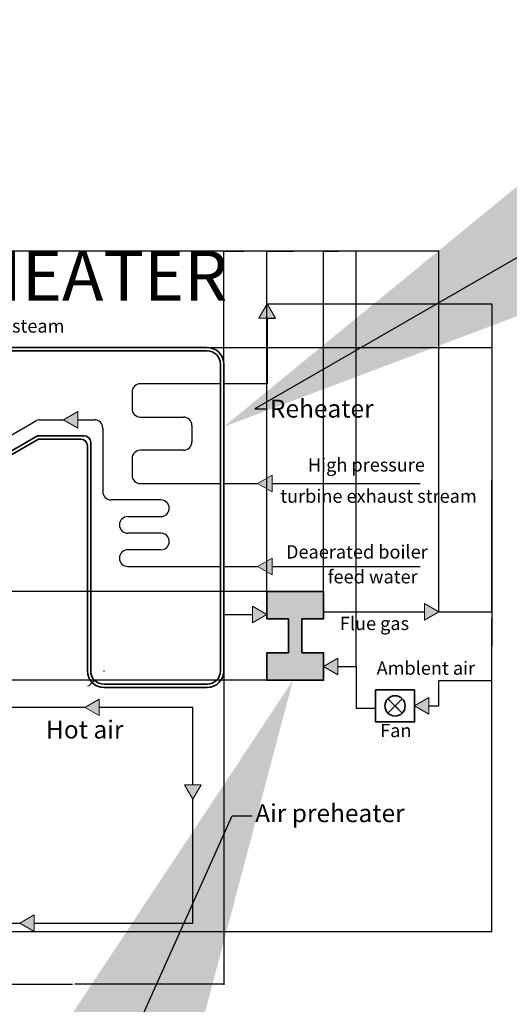
# Model space of a CAD drawing. Units: inches. Extents: x -9413 to 9703, y -9719 to 9096.
# Tile 1 of 1: x 159.8 to 307, y -19.4 to 276.8. Entities that reach past the tile are written whole.
import ezdxf
from ezdxf import colors
from ezdxf.entities.mleader import LeaderData, LeaderLine
from ezdxf.math import Vec2, Vec3

# ---------------------------------------------------------------- set-up
doc = ezdxf.new("R2010")
doc.units = ezdxf.units.IN
doc.header["$MEASUREMENT"] = 0
for name, color, linetype, lineweight in [('M-ANNO-TEXT', 7, 'Continuous', 18), ('M-ANNO-TITL', 7, 'Continuous', 35), ('M-DIMS', 2, 'Continuous', 18), ('M-DUCT-AIR', 4, 'Continuous', 25), ('M-DUCT-FLUE', 8, 'Continuous', 25), ('M-EQPM', 7, 'Continuous', 35), ('M-EQPM-PATT', 252, 'Continuous', 13), ('M-FLOW-PATT', 252, 'Continuous', 13), ('M-FLOW-SYMB', 7, 'Continuous', 18), ('M-PIPE-BWTR', 151, 'Continuous', 25), ('M-PIPE-STEM', 1, 'Continuous', 25)]:
    doc.layers.add(name, color=color, linetype=linetype, lineweight=lineweight)
doc.styles.get("Standard").update_dxf_attribs({"font": 'arial.ttf'})
doc.dimstyles.get("Standard").update_dxf_attribs({"dimtxt": 0.18, "dimasz": 0.18, "dimexe": 0.18, "dimexo": 0.0625, "dimgap": 0.09, "dimtad": 0, "dimtih": 1, "dimtoh": 1, "dimdec": 4, "dimzin": 0, "dimdsep": 46, "dimtxsty": 'Standard', "dimcen": 0.09, "dimadec": 0, "dimazin": 0, "dimtfac": 1, "dimtdec": 4, "dimtofl": 0, "dimtmove": 0, "dimatfit": 3, "dimfxl": 1, "dimtolj": 1, "dimtzin": 0, "dimarcsym": 0})

# ---------------------------------------------------------------- blocks, each defined once
blk = doc.blocks.new('FLOW-ARROW')
blk.add_lwpolyline([(0.000248294399313, -0.0003913674265164), (5.000248294399312, -0.0003913674265164), (2.500248294399312, 4.32973565149561)], close=True)
blk = doc.blocks.new('*D2')
at = {"layer": 'Defpoints', "color": 0, "transparency": 16777216}
for p in [(285.887484, 207.124736), (285.887484, 98.66208700000001), (1.37911, 71.85931899999999)]:
    blk.add_point(p, dxfattribs=at)
at = {"layer": 'M-DIMS', "color": 0, "lineweight": -2, "transparency": 16777216}
for p, q in [((1.37911, 71.921819), (1.379110000000008, 207.304736)), ((1.559110000000008, 207.124736), (143.2373829481582, 207.124736)), ((285.707484, 207.124736), (144.0292110518417, 207.124736)), ((285.887484, 98.72458700000001), (285.887484, 207.304736))]:
    blk.add_line(p, q, dxfattribs=at)
at = {"layer": 'M-DIMS', "color": 0, "transparency": 16777216}
for points in [[(1.559110000000008, 207.154736), (1.559110000000008, 207.094736), (1.379110000000008, 207.124736)], [(285.707484, 207.154736), (285.707484, 207.094736), (285.887484, 207.124736)]]:
    blk.add_solid(points, dxfattribs=at)
at = {"layer": 'M-DIMS', "color": 0, "transparency": 16777216, "insert": (143.633297, 207.124736), "char_height": 0.18, "attachment_point": 5}
blk.add_mtext('\\A1;284.5', dxfattribs=at)
blk = doc.blocks.new('*D3')
at = {"layer": 'Defpoints', "color": 0, "transparency": 16777216}
for p in [(234.2342480000001, 191.274736), (44.55608500000002, 2.461023), (301.7374840000002, 2.461023000000042)]:
    blk.add_point(p, dxfattribs=at)
at = {"layer": 'M-DIMS', "color": 0, "lineweight": -2, "transparency": 16777216}
for p, q in [((234.2967480000001, 191.274736), (301.9174840000002, 191.274736)), ((301.7374840000002, 191.094736), (301.7374840000002, 97.04978263778997)), ((301.7374840000002, 2.641023000000042), (301.7374840000002, 96.68597636221016)), ((44.61858500000001, 2.461023), (301.9174840000002, 2.461023000000042))]:
    blk.add_line(p, q, dxfattribs=at)
at = {"layer": 'M-DIMS', "color": 0, "transparency": 16777216}
for points in [[(301.7074840000002, 191.094736), (301.7674840000001, 191.094736), (301.7374840000002, 191.274736)], [(301.7074840000002, 2.641023000000042), (301.7674840000002, 2.641023000000042), (301.7374840000002, 2.461023000000042)]]:
    blk.add_solid(points, dxfattribs=at)
at = {"layer": 'M-DIMS', "color": 0, "transparency": 16777216, "insert": (301.7374840000002, 96.86787949999994), "char_height": 0.18, "attachment_point": 5}
blk.add_mtext('\\A1;188.8', dxfattribs=at)
blk = doc.blocks.new('*D6')
at = {"layer": 'Defpoints', "color": 0, "transparency": 16777216}
for p in [(221.144491, 80.86084099999998), (130.910134, 46.59639499999999), (221.144491, -13.388977)]:
    blk.add_point(p, dxfattribs=at)
at = {"layer": 'M-DIMS', "color": 0, "lineweight": -2, "transparency": 16777216}
for p, q in [((221.144491, 80.798341), (221.144491, -13.568977)), ((130.910134, 46.533895), (130.910134, -13.56897699999999)), ((131.090134, -13.388977), (175.6336085436562, -13.388977)), ((220.964491, -13.388977), (176.4210164563437, -13.388977))]:
    blk.add_line(p, q, dxfattribs=at)
at = {"layer": 'M-DIMS', "color": 0, "transparency": 16777216}
for points in [[(131.090134, -13.358977), (131.090134, -13.418977), (130.910134, -13.388977)], [(220.964491, -13.358977), (220.964491, -13.418977), (221.144491, -13.388977)]]:
    blk.add_solid(points, dxfattribs=at)
at = {"layer": 'M-DIMS', "color": 0, "transparency": 16777216, "insert": (176.0273125, -13.388977), "char_height": 0.18, "attachment_point": 5}
blk.add_mtext('\\A1;90.23', dxfattribs=at)
blk = doc.blocks.new('*D11')
at = {"layer": 'Defpoints', "color": 0, "transparency": 16777216}
for p in [(234.094392, 207.124736), (234.094392, 104.790816), (221.144491, 97.87236599999999)]:
    blk.add_point(p, dxfattribs=at)
at = {"layer": 'M-DIMS', "color": 0, "lineweight": -2, "transparency": 16777216}
for p, q in [((221.144491, 97.93486600000001), (221.144491, 207.304736)), ((221.324491, 207.124736), (227.2335342694407, 207.124736)), ((233.914392, 207.124736), (228.0053487305593, 207.124736)), ((234.094392, 104.853316), (234.094392, 207.304736))]:
    blk.add_line(p, q, dxfattribs=at)
at = {"layer": 'M-DIMS', "color": 0, "transparency": 16777216}
for points in [[(221.324491, 207.154736), (221.324491, 207.094736), (221.144491, 207.124736)], [(233.914392, 207.154736), (233.914392, 207.094736), (234.094392, 207.124736)]]:
    blk.add_solid(points, dxfattribs=at)
at = {"layer": 'M-DIMS', "color": 0, "transparency": 16777216, "insert": (227.6194415, 207.124736), "char_height": 0.18, "attachment_point": 5}
blk.add_mtext('\\A1;12.95', dxfattribs=at)
blk = doc.blocks.new('*D12')
at = {"layer": 'Defpoints', "color": 0, "transparency": 16777216}
for p in [(251.162742, 207.124736), (234.094392, 104.790816), (251.162742, 104.790816)]:
    blk.add_point(p, dxfattribs=at)
at = {"layer": 'M-DIMS', "color": 0, "lineweight": -2, "transparency": 16777216}
for p, q in [((234.094392, 104.853316), (234.094392, 207.304736)), ((234.274392, 207.124736), (242.2433350763983, 207.124736)), ((250.982742, 207.124736), (243.0137989236016, 207.124736)), ((251.162742, 104.853316), (251.162742, 207.304736))]:
    blk.add_line(p, q, dxfattribs=at)
at = {"layer": 'M-DIMS', "color": 0, "transparency": 16777216}
for points in [[(234.274392, 207.154736), (234.274392, 207.094736), (234.094392, 207.124736)], [(250.982742, 207.154736), (250.982742, 207.094736), (251.162742, 207.124736)]]:
    blk.add_solid(points, dxfattribs=at)
at = {"layer": 'M-DIMS', "color": 0, "transparency": 16777216, "insert": (242.628567, 207.124736), "char_height": 0.18, "attachment_point": 5}
blk.add_mtext('\\A1;17.07', dxfattribs=at)
blk = doc.blocks.new('*D13')
at = {"layer": 'Defpoints', "color": 0, "transparency": 16777216}
for p in [(-14.47089000000002, 104.790816), (234.0943920000001, 104.790816), (234.0943920000001, 78.04556900000003)]:
    blk.add_point(p, dxfattribs=at)
at = {"layer": 'M-DIMS', "color": 0, "lineweight": -2, "transparency": 16777216}
for p, q in [((234.0318920000001, 104.790816), (-14.65089000000003, 104.790816)), ((-14.47089000000002, 104.610816), (-14.47089000000001, 91.6000956377899)), ((-14.47089000000001, 78.225569), (-14.47089000000001, 91.23628936221009)), ((234.0318920000001, 78.04556900000003), (-14.65089000000002, 78.04556899999999))]:
    blk.add_line(p, q, dxfattribs=at)
at = {"layer": 'M-DIMS', "color": 0, "transparency": 16777216}
for points in [[(-14.50089000000002, 104.610816), (-14.44089000000002, 104.610816), (-14.47089000000002, 104.790816)], [(-14.50089000000001, 78.225569), (-14.44089000000001, 78.225569), (-14.47089000000001, 78.04556899999999)]]:
    blk.add_solid(points, dxfattribs=at)
at = {"layer": 'M-DIMS', "color": 0, "transparency": 16777216, "insert": (-14.47088999999999, 91.41819249999998), "char_height": 0.18, "attachment_point": 5}
blk.add_mtext('\\A1;26.745', dxfattribs=at)
blk = doc.blocks.new('*D14')
at = {"layer": 'Defpoints', "color": 0, "transparency": 16777216}
for p in [(260.947186, 207.124736), (251.162742, 104.790816), (260.947186, 82.160223)]:
    blk.add_point(p, dxfattribs=at)
at = {"layer": 'M-DIMS', "color": 0, "lineweight": -2, "transparency": 16777216}
for p, q in [((251.162742, 104.853316), (251.162742, 207.304736)), ((251.342742, 207.124736), (255.6616283929058, 207.124736)), ((260.767186, 207.124736), (256.4482996070941, 207.124736)), ((260.947186, 82.222723), (260.947186, 207.304736))]:
    blk.add_line(p, q, dxfattribs=at)
at = {"layer": 'M-DIMS', "color": 0, "transparency": 16777216}
for points in [[(251.342742, 207.154736), (251.342742, 207.094736), (251.162742, 207.124736)], [(260.767186, 207.154736), (260.767186, 207.094736), (260.947186, 207.124736)]]:
    blk.add_solid(points, dxfattribs=at)
at = {"layer": 'M-DIMS', "color": 0, "transparency": 16777216, "insert": (256.054964, 207.124736), "char_height": 0.18, "attachment_point": 5}
blk.add_mtext('\\A1;9.784', dxfattribs=at)
blk = doc.blocks.new('*D15')
at = {"layer": 'Defpoints', "color": 0, "transparency": 16777216}
for p in [(285.8874840000001, 98.66208700000006), (285.8278400000001, 77.97123100000003), (301.7374840000002, 77.97123100000005)]:
    blk.add_point(p, dxfattribs=at)
at = {"layer": 'M-DIMS', "color": 0, "lineweight": -2, "transparency": 16777216}
for p, q in [((285.9499840000001, 98.66208700000006), (301.9174840000002, 98.66208700000008)), ((301.7374840000002, 98.48208700000006), (301.7374840000002, 88.49856213778995)), ((301.7374840000002, 78.15123100000005), (301.7374840000002, 88.13475586221016)), ((285.8903400000001, 77.97123100000003), (301.9174840000002, 77.97123100000005))]:
    blk.add_line(p, q, dxfattribs=at)
at = {"layer": 'M-DIMS', "color": 0, "transparency": 16777216}
for points in [[(301.7074840000002, 98.48208700000006), (301.7674840000002, 98.48208700000006), (301.7374840000002, 98.66208700000008)], [(301.7074840000002, 78.15123100000005), (301.7674840000002, 78.15123100000005), (301.7374840000002, 77.97123100000005)]]:
    blk.add_solid(points, dxfattribs=at)
at = {"layer": 'M-DIMS', "color": 0, "transparency": 16777216, "insert": (301.7374840000002, 88.31665899999994), "char_height": 0.18, "attachment_point": 5}
blk.add_mtext('\\A1;20.69', dxfattribs=at)
blk = doc.blocks.new('*D16')
at = {"layer": 'Defpoints', "color": 0, "transparency": 16777216}
for p in [(216.1444910000001, 178.191776), (285.8874840000001, 98.66208700000006), (301.7374840000003, 98.66208700000008)]:
    blk.add_point(p, dxfattribs=at)
at = {"layer": 'M-DIMS', "color": 0, "lineweight": -2, "transparency": 16777216}
for p, q in [((216.2069910000001, 178.191776), (301.9174840000002, 178.191776)), ((301.7374840000002, 178.011776), (301.7374840000002, 138.6088960293315)), ((301.7374840000003, 98.84208700000009), (301.7374840000002, 138.2449669706685)), ((285.9499840000001, 98.66208700000006), (301.9174840000003, 98.66208700000008))]:
    blk.add_line(p, q, dxfattribs=at)
at = {"layer": 'M-DIMS', "color": 0, "transparency": 16777216}
for points in [[(301.7074840000002, 178.011776), (301.7674840000002, 178.011776), (301.7374840000002, 178.191776)], [(301.7074840000003, 98.84208700000009), (301.7674840000002, 98.84208700000009), (301.7374840000003, 98.66208700000008)]]:
    blk.add_solid(points, dxfattribs=at)
at = {"layer": 'M-DIMS', "color": 0, "transparency": 16777216, "insert": (301.7374840000002, 138.4269314999999), "char_height": 0.18, "attachment_point": 5}
blk.add_mtext('\\A1;79.53', dxfattribs=at)
blk = doc.blocks.new('*D21')
at = {"layer": 'Defpoints', "color": 0, "transparency": 16777216}
for p in [(185.1594609999999, 80.86084099999998), (182.3312239999999, 78.03222399999994)]:
    blk.add_point(p, dxfattribs=at)
at = {"layer": 'M-DIMS', "color": 0, "lineweight": -2, "transparency": 16777216}
for p, q in [((185.0694609999999, 80.86084099999997), (185.2494609999999, 80.86084099999997)), ((185.1594609999999, 80.77084099999998), (185.1594609999999, 80.950841)), ((180.634281728986, 76.33505372897649), (182.2039533296738, 77.90493622967317)), ((180.4542817289859, 76.3350537289765), (180.634281728986, 76.33505372897649))]:
    blk.add_line(p, q, dxfattribs=at)
at = {"layer": 'M-DIMS', "color": 0, "transparency": 16777216}
blk.add_solid([(182.1827387012861, 77.92614800806084), (182.2251679580617, 77.8837244512855), (182.3312239999999, 78.03222399999994)], dxfattribs=at)
at = {"layer": 'M-DIMS', "color": 0, "transparency": 16777216, "insert": (180.026137117799, 76.33505372897649), "char_height": 0.18, "attachment_point": 5}
blk.add_mtext('\\A1;5X R4', dxfattribs=at)

msp = doc.modelspace()

# ---------------------------------------------------------------- hatches: boundary and pattern name
at = {"layer": 'M-EQPM-PATT'}
h = msp.add_hatch(color=256, dxfattribs=at)
h.set_gradient(color1=(247, 171, 174), color2=(241, 235, 31), tint=1, name='CYLINDER')
h.paths.add_polyline_path([(234.0943920106286, 104.7908162978576), (234.0943920106286, 96.56150977514116), (240.6285668506998, 96.56150977514116), (240.6285668506998, 86.27487600315693), (234.0943920106286, 86.27487600315693), (234.0943920106286, 78.04556948044049), (251.1627416907711, 78.04556948044049), (251.1627416907711, 86.27487600315693), (244.6285668506998, 86.27487600315693), (244.6285668506998, 96.56150977514116), (251.1627416907711, 96.56150977514116), (251.1627416907711, 104.7908162978576)])
h.paths.add_polyline_path([(27.22481035966126, 56.13772641082374), (15.22950676080154, 56.13772641082374), (15.22950676080154, 35.36125112538483), (27.22481035966124, 35.36125112538483)])
at = {"layer": 'M-FLOW-PATT'}
h = msp.add_hatch(color=256, dxfattribs=at)
h.set_gradient(color1=(0, 0, 255), color2=(237, 31, 36), tint=1, name='CYLINDER')
h.paths.add_polyline_path([(57.60719326604156, 174.5154936822842), (53.27706624711947, 177.0154936822843), (53.27706624711947, 172.0154936822843)])
h.paths.add_polyline_path([(104.3199532850412, 174.5154936822842), (99.98982626611915, 177.0154936822843), (99.98982626611915, 172.0154936822843)])
h.paths.add_polyline_path([(53.52042794230806, 149.5365959733167), (57.85055496123027, 147.0365959733168), (57.85055496123027, 152.0365959733167)])
h.paths.add_polyline_path([(39.53736787953737, 125.7512816544064), (42.03736787953743, 121.4211546354843), (44.53736787953743, 125.7512816544064)])
h.paths.add_polyline_path([(112.1909801989792, 134.4074487017934), (112.1909801989792, 139.4074487017932), (107.860853180057, 136.9074487017932)])
h.paths.add_polyline_path([(177.2741254076526, 153.9161106668102), (177.2741254076526, 158.9161106668101), (172.9439983887304, 156.4161106668101)])
h.paths.add_polyline_path([(49.82189913347245, 85.9441989499526), (49.82189913347245, 80.94419894995266), (54.15202615239467, 83.44419894995269)])
h.paths.add_polyline_path([(69.11352005531556, 93.50315249510626), (64.78339303639335, 96.0031524951062), (64.78339303639335, 91.00315249510626)])
h.paths.add_polyline_path([(69.11352005531553, 73.38524540479911), (64.78339303639335, 75.885245404799), (64.78339303639335, 70.88524540479908)])
h.paths.add_polyline_path([(18.72715856023135, 60.46785342974584), (21.22715856023142, 56.13772641082373), (23.72715856023141, 60.46785342974583)])
h.paths.add_polyline_path([(21.22715856023142, 35.36125112538483), (18.72715856023142, 31.0311241064627), (23.72715856023143, 31.03112410646267)])
h.paths.add_polyline_path([(44.55608540223805, 7.461022688866137), (40.22595838331583, 4.961022688866137), (44.55608540223805, 2.461022688866222)])
h.paths.add_polyline_path([(98.78154953768238, 2.461022688866194), (98.78154953768238, 7.461022688866137), (94.45142251876013, 4.961022688866108)])
h.paths.add_polyline_path([(97.51182696160306, 19.53928695608056), (100.0118269616031, 15.20915993715846), (102.5118269616031, 19.53928695608053)])
h.paths.add_polyline_path([(164.1352451136813, 2.461022688866222), (164.1352451136813, 7.461022688866108), (159.8051180947591, 4.961022688866165)])
h.paths.add_polyline_path([(209.3801796746353, 46.61055823726996), (211.8801796746354, 42.28043121834784), (214.3801796746354, 46.61055823726991)])
h.paths.add_polyline_path([(183.686965899029, 72.398812257232), (179.3568388801068, 69.89881225723198), (183.686965899029, 67.3988122572321)])
h.paths.add_polyline_path([(130.9101338678906, 88.12957450655973), (135.2402608868128, 85.6295745065598), (135.2402608868128, 90.62957450655973)])
h.paths.add_polyline_path([(235.6787428099642, 114.793018678795), (231.348615791042, 112.293018678795), (235.6787428099642, 109.7930186787951)])
h.paths.add_polyline_path([(234.0943920106286, 97.87236613613993), (229.7642649917063, 100.3723661361398), (229.7642649917063, 95.37236613613992)])
h.paths.add_polyline_path([(235.6787428099642, 139.7381753554388), (231.348615791042, 137.2381753554388), (235.6787428099642, 134.7381753554389)])
h.paths.add_polyline_path([(234.2342482943993, 191.2747356514956), (231.7342482943993, 186.9446086325734), (236.7342482943993, 186.9446086325734)])
h.paths.add_polyline_path([(281.5573566069943, 96.1620867934123), (285.8874836259165, 98.6620867934123), (281.5573566069943, 101.1620867934122)])
h.paths.add_polyline_path([(282.8693181059843, 72.82025870979582), (278.539191087062, 70.32025870979582), (282.8693181059843, 67.8202587097959)])
h.paths.add_polyline_path([(255.4928687096933, 79.6602227417988), (255.4928687096933, 84.66022274179872), (251.1627416907711, 82.16022274179872)])

# ---------------------------------------------------------------- linework, layer by layer
at = {"layer": 'M-DUCT-AIR'}
for p, q in [((255.4928687096933, 82.16022274179872), (260.947185755821, 82.16022274179872)), ((260.947185755821, 82.16022274179872), (260.947185755821, 69.69865774240094)), ((285.8278402496623, 70.3202587097958), (285.8278402496623, 77.9712308323052)), ((179.3568388801068, 69.898812257232), (151.2395643983297, 69.898812257232)), ((211.8801796746354, 69.89881225723201), (183.686965899029, 69.89881225723201)), ((211.8801796746354, 46.61055823726992), (211.8801796746354, 69.89881225723201)), ((260.947185755821, 69.69865774240094), (266.796109151637, 69.69865774240094)), ((282.8693181059843, 70.3202587097958), (285.8278402496623, 70.3202587097958)), ((211.8801796746354, 4.961022688866137), (211.8801796746354, 42.28043121834781)), ((98.78154953768238, 4.961022688866137), (159.8051180947591, 4.961022688866137)), ((164.1352451136813, 4.961022688866137), (211.8801796746354, 4.961022688866137))]:
    msp.add_line(p, q, dxfattribs=at)
at = {"layer": 'M-DUCT-FLUE'}
for p, q in [((221.144491006682, 97.87236613613992), (229.7642649917063, 97.87236613613992)), ((251.1627416907711, 98.66208679341224), (281.5573566069943, 98.66208679341224))]:
    msp.add_line(p, q, dxfattribs=at)
at = {"layer": 'M-EQPM'}
for p, q in [((240.6285668506998, 96.56150977514116), (240.6285668506998, 86.27487600315693)), ((244.6285668506998, 96.56150977514116), (244.6285668506998, 86.27487600315693)), ((274.8284393526801, 68.15946947646528), (270.5068608860191, 72.48104794312637)), ((272.6676501193495, 70.3202587097958), (274.8284393526801, 72.48104794312636)), ((272.6676501193495, 70.32025870979582), (270.506860886019, 68.15946947646528)), ((272.6676501193495, 70.3202587097958), (274.8284393526801, 68.15946947646528))]:
    msp.add_line(p, q, dxfattribs=at)
for points in [[(133.4101338678906, 132.1038932309546), (165.458308006557, 150.6069151969495), (178.1594605795933, 150.6069151969495, -0.4142135623730951), (180.1594605795933, 148.6069151969495), (180.1594605795933, 80.86084079795216, 0.4142135623730951), (185.1594605795933, 75.86084079795216), (216.144491006682, 75.86084079795216, 0.4142135623730951), (221.144491006682, 80.86084079795216), (221.1444910066821, 173.1917761520126, 0.4142135623730951), (216.1444910066821, 178.1917761520126), (56.5363078524973, 178.1917761520126)], [(132.9101338678906, 132.969918634739), (165.1903588141258, 151.6069151969495), (179.1594605795933, 151.6069151969495, -0.4142135623730951), (181.1594605795933, 149.6069151969495), (181.1594605795933, 80.86084079795216, 0.4142135623730951), (185.1594605795933, 76.86084079795216), (216.144491006682, 76.86084079795216, 0.4142135623730951), (220.144491006682, 80.86084079795216), (220.1444910066821, 173.1917761520126, 0.4142135623730951), (216.1444910066821, 177.1917761520126), (71.38513555915277, 177.1917761520126)]]:
    msp.add_lwpolyline(points, format="xyb", dxfattribs=at)
for points in [[(240.6285668506998, 96.56150977514116), (234.0943920106286, 96.56150977514116), (234.0943920106286, 104.7908162978576), (251.1627416907711, 104.7908162978576), (251.1627416907711, 96.56150977514116), (244.6285668506998, 96.56150977514116)], [(244.6285668506998, 86.27487600315693), (251.1627416907711, 86.27487600315693), (251.1627416907711, 78.04556948044049), (234.0943920106286, 78.04556948044049), (234.0943920106286, 86.27487600315693), (240.6285668506998, 86.27487600315693)]]:
    msp.add_lwpolyline(points, dxfattribs=at)
msp.add_lwpolyline([(266.796109151637, 75.14293843849293), (278.5391910870621, 75.14293843849293), (278.5391910870621, 65.49757898109868), (266.796109151637, 65.49757898109868)], close=True, dxfattribs=at)
msp.add_circle((272.6676501193495, 70.3202587097958), 3.055817439205805, dxfattribs=at)
at = {"layer": 'M-PIPE-BWTR'}
for p, q in [((131.9759748067024, 137.2423851923322), (164.6057144799537, 156.0811741762712)), ((165.8557144799537, 156.4161106668102), (172.9439983887304, 156.4161106668102)), ((177.2741254076526, 156.4161106668102), (182.2926072427265, 156.4161106668102)), ((184.7926072427265, 153.9161106668101), (184.7926072427264, 134.793018678795)), ((202.2926072427265, 132.2930186787951), (187.2926072427264, 132.2930186787951)), ((204.7926072427265, 129.7930186787951), (204.7926072427265, 129.7930186787951)), ((189.7926072427264, 124.7930186787951), (189.7926072427264, 124.793018678795)), ((192.2926072427264, 127.293018678795), (202.2926072427265, 127.2930186787951)), ((202.2926072427265, 122.293018678795), (192.2926072427264, 122.293018678795)), ((204.7926072427265, 119.7930186787951), (204.7926072427265, 119.7930186787951)), ((202.2926072427265, 117.2930186787951), (192.2926072427265, 117.2930186787951)), ((189.7926072427265, 114.7930186787951), (189.7926072427265, 114.7930186787951)), ((192.2926072427265, 112.2930186787951), (220.144491006682, 112.2930186787951)), ((221.144491006682, 112.2930186787951), (231.348615791042, 112.2930186787951)), ((235.6787428099642, 112.2930186787951), (280.2750795346773, 112.2930186787951))]:
    msp.add_line(p, q, dxfattribs=at)
for centre, start, end in [((165.8557144799537, 153.9161106668101), 90, 120), ((182.2926072427265, 153.9161106668101), 0, 90), ((187.2926072427264, 134.793018678795), 179.9999999999999, 270), ((202.2926072427265, 129.7930186787951), 0, 90), ((202.2926072427265, 129.7930186787951), 270.0000000000001, 0), ((192.2926072427264, 124.793018678795), 90.0000000000001, 180), ((192.2926072427264, 124.7930186787951), 180, 270), ((202.2926072427265, 119.7930186787951), 0, 90), ((202.2926072427265, 119.7930186787951), 270, 0), ((192.2926072427265, 114.7930186787951), 90, 180), ((192.2926072427265, 114.7930186787951), 180, 270)]:
    msp.add_arc(centre, 2.5, start, end, dxfattribs=at)
at = {"layer": 'M-PIPE-STEM'}
for p, q in [((234.2342482943993, 186.9446086325734), (234.2342482943993, 167.2381753554389)), ((234.2342482943993, 186.9446086325734), (236.7342482943993, 186.9446086325734)), ((220.1444910066821, 167.2381753554389), (196.074814113877, 167.2381753554389)), ((234.2342482943993, 167.2381753554389), (221.1444910066821, 167.2381753554389)), ((193.574814113877, 164.7381753554389), (193.574814113877, 159.7381753554389)), ((196.074814113877, 157.2381753554389), (209.074814113877, 157.2381753554389)), ((211.574814113877, 154.7381753554389), (211.574814113877, 149.7381753554389)), ((209.074814113877, 147.2381753554389), (196.074814113877, 147.2381753554389)), ((193.574814113877, 144.7381753554389), (193.574814113877, 139.7381753554389)), ((196.074814113877, 137.2381753554389), (220.1444910066821, 137.2381753554389)), ((221.1444910066821, 137.2381753554389), (231.348615791042, 137.2381753554389)), ((235.6787428099642, 137.2381753554389), (280.2750795346774, 137.2381753554389))]:
    msp.add_line(p, q, dxfattribs=at)
for centre, start, end in [((196.074814113877, 164.7381753554389), 90, 180), ((196.074814113877, 159.7381753554389), 180, 270), ((209.074814113877, 154.7381753554389), 0, 90), ((209.074814113877, 149.7381753554389), 270, 0), ((196.074814113877, 144.7381753554389), 90, 180), ((196.074814113877, 139.7381753554389), 180, 270)]:
    msp.add_arc(centre, 2.5, start, end, dxfattribs=at)

# ---------------------------------------------------------------- block references
at = {"layer": 'M-FLOW-SYMB'}
msp.add_blockref('FLOW-ARROW', (231.734, 186.945), dxfattribs=at)
for p, rotation in [((177.2745361206232, 158.9158958798761), 210.0000000000003), ((235.6791535229349, 139.7379605685048), 210.0000000000003), ((235.6791535229349, 114.7928038918611), 210.0000000000004), ((229.7638542787357, 95.37258092307387), 30.00000000000097), ((281.5569458940236, 96.16230158034628), 30.00000000000043), ((255.4932794226639, 84.66000795486474), 210.0000000000003), ((183.6873766119997, 72.398597470298), 209.9999999999999), ((282.869728818955, 72.82004392286188), 210.0000000000004), ((214.3804279690347, 46.61016686984334), 180), ((164.135655826652, 7.460807901932128), 210)]:
    msp.add_blockref('FLOW-ARROW', p, dxfattribs=dict(at, rotation=rotation))

# ---------------------------------------------------------------- texts
at = {"layer": 'M-ANNO-TEXT', "attachment_point": 1}
for s, width, heights, insert, char_height in [('Superheated steam', 70.22066543495748, [13.99584833657717], (123.307481320051, 186.6375065489846), 4), ('High pressure', 47.30068486416712, [0], (246.476169417554, 144.8458649818801), 4), ('turbine exhaust stream', 64.11546079284744, [0], (238.1527707168134, 135.447721903534), 4), ('Deaerated boiler', 43.33689305087318, [0], (239.8820720470976, 118.6797881484833), 4), ('feed water', 27.50805079104612, [0], (252.4011732143117, 111.1916892744354), 4), ('Flue gas', 27.35668208095012, [0], (256.0710026049055, 97.14541449309189), 4), ('Amblent air', 33.15350823279004, [0], (267.1375282618101, 83.70583816718135), 4), ('Hot air', 27.52518381383822, [0], (167.7190620238642, 65.91979562440329), 5.4), ('Fan', 10.96373282681452, [0], (268.194576078812, 64.92952374547274), 4)]:
    msp.add_mtext_dynamic_manual_height_columns(s, width=width, gutter_width=1, heights=heights, dxfattribs=dict(at, insert=insert, char_height=char_height))
at = {"layer": 'M-ANNO-TITL', "insert": (71.55599227099447, 207.2732170699019), "char_height": 15, "attachment_point": 1}
msp.add_mtext_dynamic_manual_height_columns('AIR PREHEATER', width=207.9937702218885, gutter_width=1, heights=[0], dxfattribs=at)

# ---------------------------------------------------------------- dimensions: what is measured, and where the dimension line sits
at = {"layer": 'M-DIMS'}
for base, p1, p2, override, picture, middle in [((285.887484, 207.124736), (1.37911, 71.85931899999999), (285.887484, 98.66208700000001), {"dimdec": 1, "dimlfac": 1, "dimrnd": 0, "dimzin": 0, "dimdsep": 46, "dimlunit": 2}, '*D2', (143.633297, 207.124736)), ((234.094392, 207.124736), (221.144491, 97.87236599999999), (234.094392, 104.790816), {"dimdec": 2, "dimlfac": 1, "dimrnd": 0, "dimzin": 0, "dimdsep": 46, "dimlunit": 2}, '*D11', (227.6194415, 207.124736)), ((251.162742, 207.124736), (234.094392, 104.790816), (251.162742, 104.790816), {"dimdec": 2, "dimlfac": 1, "dimrnd": 0, "dimzin": 0, "dimdsep": 46, "dimlunit": 2}, '*D12', (242.628567, 207.124736)), ((260.947186, 207.124736), (251.162742, 104.790816), (260.947186, 82.160223), {"dimdec": 3, "dimlfac": 1, "dimrnd": 0, "dimzin": 0, "dimdsep": 46, "dimlunit": 2}, '*D14', (256.054964, 207.124736)), ((221.144491, -13.388977), (130.910134, 46.59639499999999), (221.144491, 80.86084099999998), {"dimdec": 2, "dimlfac": 1, "dimrnd": 0, "dimzin": 0, "dimdsep": 46, "dimlunit": 2}, '*D6', (176.0273125, -13.388977))]:
    dim = msp.add_linear_dim(base=base, p1=p1, p2=p2, dimstyle='Standard', override=override, dxfattribs=at)
    dim.commit()
    dim.dimension.update_dxf_attribs({"geometry": picture, "text_midpoint": middle})
for base, p1, p2, override, picture, middle in [((301.7374840000002, 2.461023000000042), (234.234248, 191.274736), (44.556085, 2.461022999999999), {"dimdec": 1, "dimlfac": 1, "dimrnd": 0, "dimzin": 0, "dimdsep": 46, "dimlunit": 2}, '*D3', (301.7374840000002, 96.86787949999994)), ((301.7374840000003, 98.66208700000008), (216.144491, 178.191776), (285.887484, 98.66208700000001), {"dimdec": 2, "dimlfac": 1, "dimrnd": 0, "dimzin": 0, "dimdsep": 46, "dimlunit": 2}, '*D16', (301.7374840000002, 138.4269314999999)), ((-14.47089000000002, 104.790816), (234.094392, 78.045569), (234.094392, 104.790816), {"dimdec": 3, "dimlfac": 1, "dimrnd": 0, "dimzin": 0, "dimdsep": 46, "dimlunit": 2}, '*D13', (-14.47088999999999, 91.41819249999998)), ((301.7374840000002, 77.97123100000005), (285.887484, 98.66208700000001), (285.82784, 77.971231), {"dimdec": 2, "dimlfac": 1, "dimrnd": 0, "dimzin": 0, "dimdsep": 46, "dimlunit": 2}, '*D15', (301.7374840000002, 88.31665899999994))]:
    dim = msp.add_linear_dim(base=base, p1=p1, p2=p2, angle=90, dimstyle='Standard', override=override, dxfattribs=at)
    dim.commit()
    dim.dimension.update_dxf_attribs({"geometry": picture, "text_midpoint": middle})
dim = msp.add_radius_dim(center=(185.1594609999999, 80.86084099999998), mpoint=(182.3312239999999, 78.03222399999994), text='5X <>', dimstyle='Standard', override={"dimdec": 0, "dimlfac": 1, "dimrnd": 0, "dimzin": 0, "dimdsep": 46, "dimlunit": 2}, dxfattribs=at)
dim.commit()
dim.dimension.update_dxf_attribs({"geometry": '*D21', "text_midpoint": (180.026137117799, 76.33505372897649), "dimtype": 164})

# ---------------------------------------------------------------- leaders
at = {"layer": 'M-ANNO-TEXT'}
ml = msp.add_multileader_mtext('Standard', dxfattribs=at)
ml.set_content('Reheater', color=256)
ml.set_leader_properties()
ml.build(insert=Vec2(0, 0))
ml.multileader.update_dxf_attribs({"dogleg_length": 0.36, "arrow_head_size": 10000, "scale": 10})
ctx = ml.context
ctx.base_point, ctx.scale, ctx.char_height, ctx.arrow_head_size, ctx.landing_gap_size, ctx.plane_origin = Vec3(234.1414050860131, 159.7303554673012), 10, 5.4, 10000, 0.9, Vec3(221.1444910066821, 154.3050445940477)
notes = []
notes.append((ctx, [(0, (1, 1, 0), (230.5414050860131, 159.7303554673012), (1, 0), 3.599999999999999, [(0, [(221.1444910066821, 154.3050445940477)], 0, [])])]))
ctx.mtext.insert, ctx.mtext.flow_direction = Vec3(235.0414050860131, 162.4745573772603), 5
ml = msp.add_multileader_mtext('Standard', dxfattribs=at)
ml.set_content('Air preheater', color=256)
ml.set_leader_properties()
ml.build(insert=Vec2(0, 0))
ml.multileader.update_dxf_attribs({"dogleg_length": 0.36, "arrow_head_size": 10000, "scale": 10})
ctx = ml.context
ctx.base_point, ctx.scale, ctx.char_height, ctx.arrow_head_size, ctx.landing_gap_size, ctx.plane_origin = Vec3(229.7079293124727, 37.30650895205824), 10, 5.4, 10000, 0.9, Vec3(241.9833706008503, 78.04556948044049)
notes.append((ctx, [(1, (1, 1, 0), (223.7048975654645, 37.30650895205824), (1, 0), 6.003031747008185, [(0, [(241.9833706008503, 78.04556948044049)], 0, [])])]))
ctx.mtext.insert, ctx.mtext.flow_direction = Vec3(230.6079293124727, 40.75609967511417), 5
for ctx, leaders in notes:
    for number, flags, end, landing, length, lines in leaders:
        leader = LeaderData()
        leader.index, (leader.has_last_leader_line, leader.has_dogleg_vector, leader.attachment_direction) = number, flags
        leader.last_leader_point, leader.dogleg_vector, leader.dogleg_length = Vec3(end), Vec3(landing), length
        for number, points, colour, breaks in lines:
            line = LeaderLine()
            line.index, line.vertices, line.color, line.breaks = number, Vec3.list(points), colors.encode_raw_color(colour), breaks
            leader.lines.append(line)
        ctx.leaders.append(leader)

doc.saveas('drawing.dxf')
